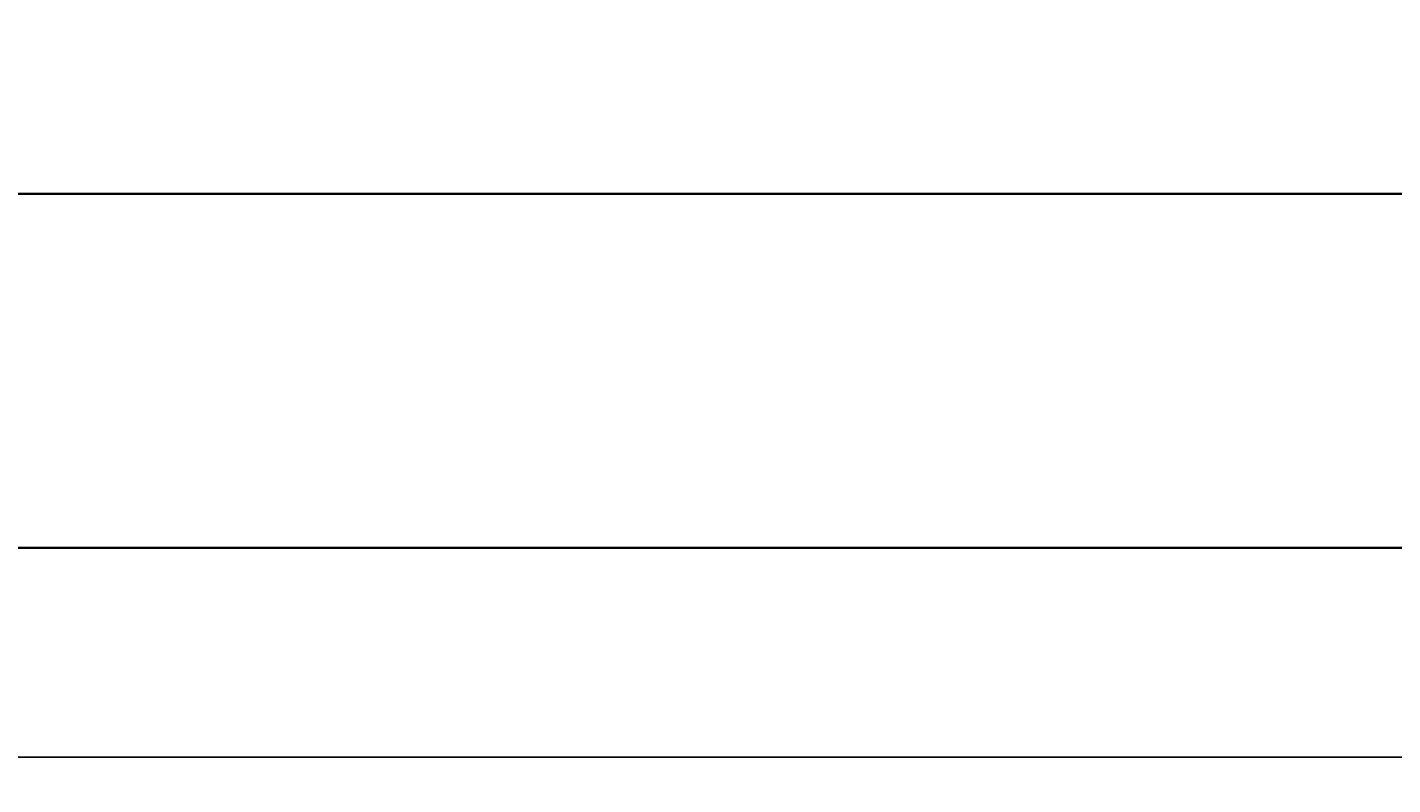
# Model space of a CAD drawing. Units: inches. Extents: x -61 to 1599, y -1316 to 257.
# Tile 46 of 204: x 114 to 149, y -447 to -428. Entities that reach past the tile are written whole.
import ezdxf

# ---------------------------------------------------------------- set-up
doc = ezdxf.new("R2010")
doc.units = ezdxf.units.IN
doc.header["$MEASUREMENT"] = 0
doc.layers.add('A-ANNO-DIMS', color=2, linetype='Continuous', lineweight=18)
doc.layers.add('WALLS', color=4, linetype='Continuous', lineweight=35)
doc.styles.get("Standard").update_dxf_attribs({"font": 'arial.ttf'})
doc.dimstyles.get("Standard").update_dxf_attribs({"dimtxt": 0.18, "dimasz": 0.18, "dimexe": 0.18, "dimexo": 0.0625, "dimgap": 0.09, "dimtad": 0, "dimtih": 1, "dimtoh": 1, "dimdec": 0, "dimzin": 0, "dimdsep": 46, "dimlunit": 3, "dimtxsty": 'Standard', "dimcen": 0.09, "dimadec": 0, "dimazin": 0, "dimtfac": 1, "dimtdec": 0, "dimtofl": 0, "dimtmove": 0, "dimatfit": 3, "dimfxl": 1, "dimtolj": 1, "dimtzin": 0, "dimarcsym": 0})

# ---------------------------------------------------------------- blocks, each defined once
blk = doc.blocks.new('*D687')
at = {"layer": 'A-ANNO-DIMS', "color": 0, "lineweight": -2, "transparency": 16777216}
for p, q in [((289.418, 181.677), (-61.077, 181.677)), ((-60.897, 181.497), (-60.897, -528.952)), ((-60.897, -1239.765), (-60.897, -529.316)), ((319.64, -1239.945), (-61.077, -1239.945))]:
    blk.add_line(p, q, dxfattribs=at)
at = {"layer": 'A-ANNO-DIMS', "color": 0, "transparency": 16777216}
for points in [[(-60.927, 181.497), (-60.867, 181.497), (-60.897, 181.677)], [(-60.927, -1239.765), (-60.867, -1239.765), (-60.897, -1239.945)]]:
    blk.add_solid(points, dxfattribs=at)
at = {"layer": 'DEFPOINTS', "color": 0, "transparency": 16777216}
for p in [(289.481, 181.677), (-60.897, -1239.945), (319.703, -1239.945)]:
    blk.add_point(p, dxfattribs=at)
at = {"layer": 'A-ANNO-DIMS', "color": 0, "transparency": 16777216, "insert": (-60.897, -529.134), "char_height": 0.18, "attachment_point": 5}
blk.add_mtext('\\A1;1421.6', dxfattribs=at)
blk = doc.blocks.new('*D699')
at = {"layer": 'A-ANNO-DIMS', "color": 0, "lineweight": -2, "transparency": 16777216}
for p, q in [((835.64, -167.169), (-61.077, -167.169)), ((-60.897, -167.349), (-60.897, -306.726)), ((-60.897, -446.466), (-60.897, -307.09)), ((841.64, -446.646), (-61.077, -446.646))]:
    blk.add_line(p, q, dxfattribs=at)
at = {"layer": 'A-ANNO-DIMS', "color": 0, "transparency": 16777216}
for points in [[(-60.927, -167.349), (-60.867, -167.349), (-60.897, -167.169)], [(-60.927, -446.466), (-60.867, -446.466), (-60.897, -446.646)]]:
    blk.add_solid(points, dxfattribs=at)
at = {"layer": 'DEFPOINTS', "color": 0, "transparency": 16777216}
for p in [(835.703, -167.169), (-60.897, -446.646), (841.703, -446.646)]:
    blk.add_point(p, dxfattribs=at)
at = {"layer": 'A-ANNO-DIMS', "color": 0, "transparency": 16777216, "insert": (-60.897, -306.908), "char_height": 0.18, "attachment_point": 5}
blk.add_mtext('\\A1;279.5', dxfattribs=at)
blk = doc.blocks.new('*D700')
at = {"layer": 'A-ANNO-DIMS', "color": 0, "lineweight": -2, "transparency": 16777216}
for p, q in [((14.703, -616.882), (14.703, 257.457)), ((14.883, 257.277), (96.772, 257.277)), ((179.572, 257.277), (97.683, 257.277)), ((179.752, -616.882), (179.752, 257.457))]:
    blk.add_line(p, q, dxfattribs=at)
at = {"layer": 'A-ANNO-DIMS', "color": 0, "transparency": 16777216}
for points in [[(14.883, 257.307), (14.883, 257.247), (14.703, 257.277)], [(179.572, 257.307), (179.572, 257.247), (179.752, 257.277)]]:
    blk.add_solid(points, dxfattribs=at)
at = {"layer": 'DEFPOINTS', "color": 0, "transparency": 16777216}
for p in [(179.752, 257.277), (14.703, -616.945), (179.752, -616.945)]:
    blk.add_point(p, dxfattribs=at)
at = {"layer": 'A-ANNO-DIMS', "color": 0, "transparency": 16777216, "insert": (97.227, 257.277), "char_height": 0.18, "attachment_point": 5}
blk.add_mtext('\\A1;165.05', dxfattribs=at)

msp = doc.modelspace()

# ---------------------------------------------------------------- linework, layer by layer
at = {"layer": 'WALLS'}
for p, q in [((87.7028, -432.3229), (237.7028, -432.3229)), ((14.7028, -441.3229), (237.7028, -441.3229))]:
    msp.add_line(p, q, dxfattribs=at)

# ---------------------------------------------------------------- dimensions: what is measured, and where the dimension line sits
at = {"layer": 'A-ANNO-DIMS'}
dim = msp.add_linear_dim(base=(179.7521, 257.2771), p1=(14.7028, -616.9446), p2=(179.7521, -616.9446), dimstyle='Standard', override={"dimdec": 2, "dimlfac": 1, "dimrnd": 0, "dimzin": 0, "dimdsep": 46, "dimlunit": 2}, dxfattribs=at)
dim.commit()
dim.dimension.update_dxf_attribs({"geometry": '*D700', "text_midpoint": (97.2274, 257.2771)})
for base, p1, p2, picture, middle in [((-60.8972, -1239.9446), (289.4807, 181.6771), (319.7028, -1239.9446), '*D687', (-60.8972, -529.1337)), ((-60.8972, -446.6462), (835.7028, -167.169), (841.7028, -446.6462), '*D699', (-60.8972, -306.9076))]:
    dim = msp.add_linear_dim(base=base, p1=p1, p2=p2, angle=90, dimstyle='Standard', override={"dimdec": 1, "dimlfac": 1, "dimrnd": 0, "dimzin": 0, "dimdsep": 46, "dimlunit": 2}, dxfattribs=at)
    dim.commit()
    dim.dimension.update_dxf_attribs({"geometry": picture, "text_midpoint": middle})

doc.saveas('drawing.dxf')
